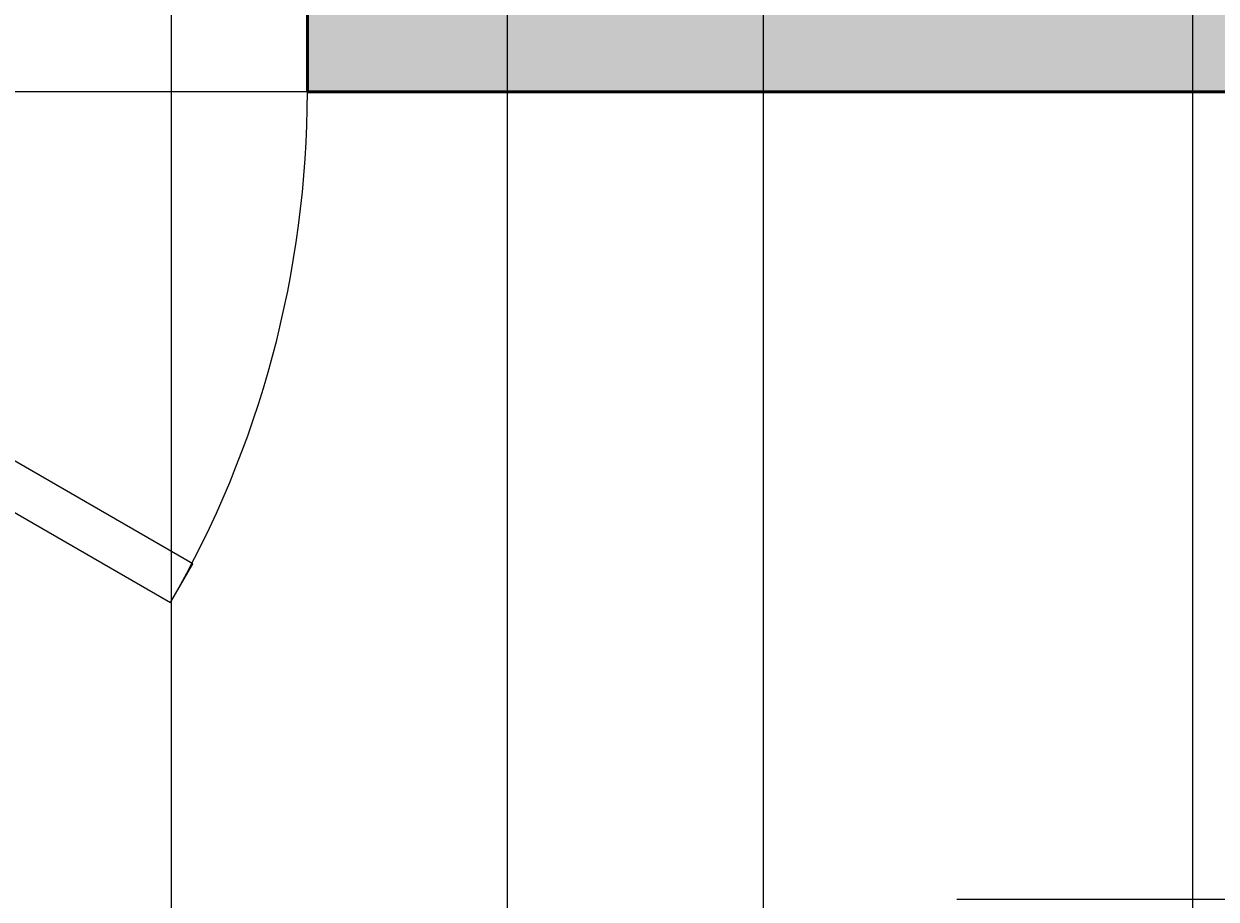
# Model space of a CAD drawing. Units: inches. Extents: x 2231 to 2461, y 2045 to 2455.
# Tile 27 of 95: x 2326 to 2361, y 2159 to 2185. Entities that reach past the tile are written whole.
import ezdxf

# ---------------------------------------------------------------- set-up
doc = ezdxf.new("R2010")
doc.units = ezdxf.units.IN
for name, color, linetype, lineweight in [('A-ANNO-DIMS', 2, 'Continuous', 18), ('A-DOOR', 3, 'Continuous', 25), ('A-WALL', 7, 'Continuous', 50)]:
    doc.layers.add(name, color=color, linetype=linetype, lineweight=lineweight)
doc.layers.add('A-WALL-PATT', color=18, linetype='Continuous', lineweight=13, true_color=0x000000)
doc.styles.get("Standard").update_dxf_attribs({"font": 'arial.ttf'})
doc.dimstyles.get("Standard").update_dxf_attribs({"dimtxt": 0.18, "dimasz": 0.18, "dimexe": 0.18, "dimexo": 0.0625, "dimgap": 0.09, "dimtad": 0, "dimtih": 1, "dimtoh": 1, "dimdec": 4, "dimzin": 0, "dimdsep": 46, "dimtxsty": 'Standard', "dimcen": 0.09, "dimadec": 0, "dimazin": 0, "dimtfac": 1, "dimtdec": 4, "dimtofl": 0, "dimtmove": 0, "dimatfit": 3, "dimfxl": 1, "dimtolj": 1, "dimtzin": 0, "dimarcsym": 0})

# ---------------------------------------------------------------- blocks, each defined once
blk = doc.blocks.new('*U4')
for p, q in [((0, 0), (0, 6)), ((40, 0), (40, 6))]:
    blk.add_line(p, q)
blk.add_lwpolyline([(0, 0), (34.641, -20), (35.516, -18.484), (0.875, 1.516)], close=True)
blk.add_arc((0, 0), 40, 330, 0)
blk = doc.blocks.new('*D50')
at = {"layer": 'A-ANNO-DIMS', "color": 0, "lineweight": -2, "transparency": 16777216}
for p, q in [((2304.794, 2182.895), (2304.794, 2454.645)), ((2334.794, 2182.895), (2334.794, 2454.645)), ((2304.974, 2454.465), (2319.575, 2454.465)), ((2334.614, 2454.465), (2320.012, 2454.465))]:
    blk.add_line(p, q, dxfattribs=at)
at = {"layer": 'A-ANNO-DIMS', "color": 0, "transparency": 16777216}
for points in [[(2304.974, 2454.495), (2304.974, 2454.435), (2304.794, 2454.465)], [(2334.614, 2454.495), (2334.614, 2454.435), (2334.794, 2454.465)]]:
    blk.add_solid(points, dxfattribs=at)
at = {"layer": 'Defpoints', "color": 0, "transparency": 16777216}
for p in [(2334.794, 2454.465), (2304.794, 2182.833), (2334.794, 2182.833)]:
    blk.add_point(p, dxfattribs=at)
at = {"layer": 'A-ANNO-DIMS', "color": 0, "transparency": 16777216, "insert": (2319.794, 2454.465), "char_height": 0.18, "attachment_point": 5}
blk.add_mtext('\\A1;30', dxfattribs=at)
blk = doc.blocks.new('*D51')
at = {"layer": 'A-ANNO-DIMS', "color": 0, "lineweight": -2, "transparency": 16777216}
for p, q in [((2258.794, 2306.77), (2258.794, 2044.803)), ((2330.794, 2306.77), (2330.794, 2044.803)), ((2258.974, 2044.983), (2294.576, 2044.983)), ((2330.614, 2044.983), (2295.011, 2044.983))]:
    blk.add_line(p, q, dxfattribs=at)
at = {"layer": 'A-ANNO-DIMS', "color": 0, "transparency": 16777216}
for points in [[(2258.974, 2045.013), (2258.974, 2044.953), (2258.794, 2044.983)], [(2330.614, 2045.013), (2330.614, 2044.953), (2330.794, 2044.983)]]:
    blk.add_solid(points, dxfattribs=at)
at = {"layer": 'Defpoints', "color": 0, "transparency": 16777216}
for p in [(2258.794, 2306.833), (2330.794, 2306.833), (2330.794, 2044.983)]:
    blk.add_point(p, dxfattribs=at)
at = {"layer": 'A-ANNO-DIMS', "color": 0, "transparency": 16777216, "insert": (2294.794, 2044.983), "char_height": 0.18, "attachment_point": 5}
blk.add_mtext('\\A1;72', dxfattribs=at)
blk = doc.blocks.new('*D52')
at = {"layer": 'A-ANNO-DIMS', "color": 0, "lineweight": -2, "transparency": 16777216}
for p, q in [((2330.794, 2306.77), (2330.794, 2044.803)), ((2360.794, 2306.77), (2360.794, 2044.803)), ((2330.974, 2044.983), (2345.575, 2044.983)), ((2360.614, 2044.983), (2346.012, 2044.983))]:
    blk.add_line(p, q, dxfattribs=at)
at = {"layer": 'A-ANNO-DIMS', "color": 0, "transparency": 16777216}
for points in [[(2330.974, 2045.013), (2330.974, 2044.953), (2330.794, 2044.983)], [(2360.614, 2045.013), (2360.614, 2044.953), (2360.794, 2044.983)]]:
    blk.add_solid(points, dxfattribs=at)
at = {"layer": 'Defpoints', "color": 0, "transparency": 16777216}
for p in [(2330.794, 2306.833), (2360.794, 2306.833), (2360.794, 2044.983)]:
    blk.add_point(p, dxfattribs=at)
at = {"layer": 'A-ANNO-DIMS', "color": 0, "transparency": 16777216, "insert": (2345.794, 2044.983), "char_height": 0.18, "attachment_point": 5}
blk.add_mtext('\\A1;30', dxfattribs=at)
blk = doc.blocks.new('*D60')
at = {"layer": 'A-ANNO-DIMS', "color": 0, "lineweight": -2, "transparency": 16777216}
for p, q in [((2432.731, 2182.833), (2230.981, 2182.833)), ((2231.161, 2182.653), (2231.161, 2166.906)), ((2231.161, 2150.795), (2231.161, 2166.542)), ((2432.731, 2150.615), (2230.981, 2150.615))]:
    blk.add_line(p, q, dxfattribs=at)
at = {"layer": 'A-ANNO-DIMS', "color": 0, "transparency": 16777216}
for points in [[(2231.131, 2182.653), (2231.191, 2182.653), (2231.161, 2182.833)], [(2231.131, 2150.795), (2231.191, 2150.795), (2231.161, 2150.615)]]:
    blk.add_solid(points, dxfattribs=at)
at = {"layer": 'Defpoints', "color": 0, "transparency": 16777216}
for p in [(2231.161, 2182.833), (2432.794, 2182.833), (2432.794, 2150.615)]:
    blk.add_point(p, dxfattribs=at)
at = {"layer": 'A-ANNO-DIMS', "color": 0, "transparency": 16777216, "insert": (2231.161, 2166.724), "char_height": 0.18, "attachment_point": 5}
blk.add_mtext('\\A1;32.22', dxfattribs=at)
blk = doc.blocks.new('*D65')
at = {"layer": 'A-ANNO-DIMS', "color": 0, "lineweight": -2, "transparency": 16777216}
for p, q in [((2285.635, 2189.285), (2285.635, 2044.803)), ((2340.667, 2189.285), (2340.667, 2044.803)), ((2285.815, 2044.983), (2312.758, 2044.983)), ((2340.487, 2044.983), (2313.545, 2044.983))]:
    blk.add_line(p, q, dxfattribs=at)
at = {"layer": 'A-ANNO-DIMS', "color": 0, "transparency": 16777216}
for points in [[(2285.815, 2045.013), (2285.815, 2044.953), (2285.635, 2044.983)], [(2340.487, 2045.013), (2340.487, 2044.953), (2340.667, 2044.983)]]:
    blk.add_solid(points, dxfattribs=at)
at = {"layer": 'Defpoints', "color": 0, "transparency": 16777216}
for p in [(2285.635, 2189.348), (2340.667, 2189.348), (2340.667, 2044.983)]:
    blk.add_point(p, dxfattribs=at)
at = {"layer": 'A-ANNO-DIMS', "color": 0, "transparency": 16777216, "insert": (2313.151, 2044.983), "char_height": 0.18, "attachment_point": 5}
blk.add_mtext('\\A1;55.03', dxfattribs=at)
blk = doc.blocks.new('*D66')
at = {"layer": 'A-ANNO-DIMS', "color": 0, "lineweight": -2, "transparency": 16777216}
for p, q in [((2348.189, 2096.895), (2348.189, 2454.645)), ((2408.794, 2096.895), (2408.794, 2454.645)), ((2348.369, 2454.465), (2378.167, 2454.465)), ((2408.614, 2454.465), (2378.815, 2454.465))]:
    blk.add_line(p, q, dxfattribs=at)
at = {"layer": 'A-ANNO-DIMS', "color": 0, "transparency": 16777216}
for points in [[(2348.369, 2454.495), (2348.369, 2454.435), (2348.189, 2454.465)], [(2408.614, 2454.495), (2408.614, 2454.435), (2408.794, 2454.465)]]:
    blk.add_solid(points, dxfattribs=at)
at = {"layer": 'Defpoints', "color": 0, "transparency": 16777216}
for p in [(2408.794, 2454.465), (2348.189, 2096.833), (2408.794, 2096.833)]:
    blk.add_point(p, dxfattribs=at)
at = {"layer": 'A-ANNO-DIMS', "color": 0, "transparency": 16777216, "insert": (2378.491, 2454.465), "char_height": 0.18, "attachment_point": 5}
blk.add_mtext('\\A1;60.6', dxfattribs=at)
blk = doc.blocks.new('*D69')
at = {"layer": 'A-ANNO-DIMS', "color": 0, "lineweight": -2, "transparency": 16777216}
for p, q in [((2340.667, 2189.285), (2340.667, 2044.803)), ((2394.794, 2186.77), (2394.794, 2044.803)), ((2340.847, 2044.983), (2367.337, 2044.983)), ((2394.614, 2044.983), (2368.124, 2044.983))]:
    blk.add_line(p, q, dxfattribs=at)
at = {"layer": 'A-ANNO-DIMS', "color": 0, "transparency": 16777216}
for points in [[(2340.847, 2045.013), (2340.847, 2044.953), (2340.667, 2044.983)], [(2394.614, 2045.013), (2394.614, 2044.953), (2394.794, 2044.983)]]:
    blk.add_solid(points, dxfattribs=at)
at = {"layer": 'Defpoints', "color": 0, "transparency": 16777216}
for p in [(2340.667, 2189.348), (2394.794, 2186.833), (2394.794, 2044.983)]:
    blk.add_point(p, dxfattribs=at)
at = {"layer": 'A-ANNO-DIMS', "color": 0, "transparency": 16777216, "insert": (2367.73, 2044.983), "char_height": 0.18, "attachment_point": 5}
blk.add_mtext('\\A1;54.13', dxfattribs=at)
blk = doc.blocks.new('*D73')
at = {"layer": 'A-ANNO-DIMS', "color": 0, "lineweight": -2, "transparency": 16777216}
for p, q in [((2334.856, 2182.833), (2460.606, 2182.833)), ((2460.426, 2182.653), (2460.426, 2171.156)), ((2460.426, 2159.295), (2460.426, 2170.792)), ((2353.872, 2159.115), (2460.606, 2159.115))]:
    blk.add_line(p, q, dxfattribs=at)
at = {"layer": 'A-ANNO-DIMS', "color": 0, "transparency": 16777216}
for points in [[(2460.396, 2182.653), (2460.456, 2182.653), (2460.426, 2182.833)], [(2460.396, 2159.295), (2460.456, 2159.295), (2460.426, 2159.115)]]:
    blk.add_solid(points, dxfattribs=at)
at = {"layer": 'Defpoints', "color": 0, "transparency": 16777216}
for p in [(2334.794, 2182.833), (2460.426, 2182.833), (2353.809, 2159.115)]:
    blk.add_point(p, dxfattribs=at)
at = {"layer": 'A-ANNO-DIMS', "color": 0, "transparency": 16777216, "insert": (2460.426, 2170.974), "char_height": 0.18, "attachment_point": 5}
blk.add_mtext('\\A1;23.717', dxfattribs=at)

msp = doc.modelspace()

# ---------------------------------------------------------------- hatches: boundary and pattern name
at = {"layer": 'A-WALL-PATT'}
h = msp.add_hatch(color=256, dxfattribs=at)
h.dxf.hatch_style = 1
h.paths.add_polyline_path([(2441.7935, 2269.1535), (2432.7935, 2269.1535), (2432.7935, 2186.8328), (2396.7935, 2186.8328), (2396.7935, 2286.8328), (2394.7935, 2286.8328), (2394.7935, 2186.8328), (2334.7935, 2186.8328), (2334.7935, 2182.8328), (2432.7935, 2182.8328), (2432.7935, 2072.8328), (2416.6639, 2072.8328), (2416.6639, 2063.8328), (2441.7935, 2063.8328)])
h.paths.add_polyline_path([(2368.6639, 2072.8328), (2367.04, 2072.8328), (2330.7942, 2072.8328), (2330.7397, 2063.8328), (2368.6639, 2063.8328)])
h.paths.add_polyline_path([(2300.7392, 2068.3328), (2300.7392, 2072.8328), (2298.7935, 2072.8328), (2294.7935, 2072.8328), (2258.7935, 2072.8328), (2258.7935, 2120.8328), (2294.7935, 2120.8328), (2298.7935, 2120.8328), (2298.7935, 2128.8328), (2294.7935, 2128.8328), (2294.7935, 2124.8328), (2258.7935, 2124.8328), (2258.7935, 2182.8328), (2294.7935, 2182.8328), (2294.7935, 2174.8328), (2298.7935, 2174.8328), (2298.7935, 2182.8328), (2304.7935, 2182.8328), (2304.7935, 2186.8328), (2258.7935, 2186.8328), (2258.7935, 2221.999), (2249.7935, 2221.999), (2249.7935, 2063.8328), (2300.7392, 2063.8328)])
h.paths.add_polyline_path([(2391.9338, 2435.8328), (2333.82, 2435.8328), (2333.82, 2426.8328), (2368.7935, 2426.8328), (2368.7935, 2374.9508), (2368.7935, 2370.8328), (2372.3935, 2370.8328), (2372.7935, 2370.8328), (2372.7935, 2426.8328), (2391.9338, 2426.8328)])
h.paths.add_polyline_path([(2441.7935, 2435.8328), (2415.9338, 2435.8328), (2415.9338, 2426.8328), (2432.7935, 2426.8328), (2432.7935, 2334.8328), (2372.7935, 2334.8328), (2372.7935, 2346.8328), (2368.7935, 2346.8328), (2368.7935, 2306.8328), (2360.7935, 2306.8328), (2360.7935, 2302.8328), (2368.7935, 2302.8328), (2372.7935, 2302.8328), (2372.7935, 2330.8328), (2432.7935, 2330.8328), (2432.7935, 2317.1535), (2441.7935, 2317.1535)])
h.paths.add_polyline_path([(2285.82, 2435.8328), (2249.7935, 2435.8328), (2249.7935, 2269.999), (2258.7935, 2269.999), (2258.7935, 2302.8328), (2318.8168, 2302.8328), (2330.7935, 2302.8328), (2330.7935, 2306.8328), (2258.7935, 2306.8328), (2258.7935, 2426.8328), (2285.82, 2426.8328)])

# ---------------------------------------------------------------- linework, layer by layer
at = {"layer": 'A-WALL'}
for q in [(2334.7935, 2186.8328), (2432.7935, 2182.8328)]:
    msp.add_line((2334.7935, 2182.8328), q, dxfattribs=at)

# ---------------------------------------------------------------- block references
at = {"layer": 'A-DOOR', "xscale": 0.75, "yscale": 0.75, "zscale": 0.75}
msp.add_blockref('*U4', (2304.7935, 2182.8328), dxfattribs=at)

# ---------------------------------------------------------------- dimensions: what is measured, and where the dimension line sits
at = {"layer": 'A-ANNO-DIMS'}
for base, p1, p2, override, picture, middle in [((2334.7935, 2454.4653), (2304.7935, 2182.8328), (2334.7935, 2182.8328), {"dimdec": 0, "dimlfac": 1, "dimrnd": 0, "dimzin": 0, "dimdsep": 46, "dimlunit": 2}, '*D50', (2319.7935, 2454.4653)), ((2408.7935, 2454.4653), (2348.1888, 2096.8328), (2408.7935, 2096.8328), {"dimdec": 1, "dimlfac": 1, "dimrnd": 0, "dimzin": 0, "dimdsep": 46, "dimlunit": 2}, '*D66', (2378.4912, 2454.4653)), ((2330.7935, 2044.9825), (2258.7935, 2306.8328), (2330.7935, 2306.8328), {"dimdec": 0, "dimlfac": 1, "dimrnd": 0, "dimzin": 0, "dimdsep": 46, "dimlunit": 2}, '*D51', (2294.7935, 2044.9825)), ((2360.7935, 2044.9825), (2330.7935, 2306.8328), (2360.7935, 2306.8328), {"dimdec": 0, "dimlfac": 1, "dimrnd": 0, "dimzin": 0, "dimdsep": 46, "dimlunit": 2}, '*D52', (2345.7935, 2044.9825)), ((2340.6673, 2044.9825), (2285.6353, 2189.3477), (2340.6673, 2189.3477), {"dimdec": 2, "dimlfac": 1, "dimrnd": 0, "dimzin": 0, "dimdsep": 46, "dimlunit": 2}, '*D65', (2313.1513, 2044.9825)), ((2394.7935, 2044.9825), (2340.6673, 2189.3477), (2394.7935, 2186.8328), {"dimdec": 2, "dimlfac": 1, "dimrnd": 0, "dimzin": 0, "dimdsep": 46, "dimlunit": 2}, '*D69', (2367.7304, 2044.9825))]:
    dim = msp.add_linear_dim(base=base, p1=p1, p2=p2, dimstyle='Standard', override=override, dxfattribs=at)
    dim.commit()
    dim.dimension.update_dxf_attribs({"geometry": picture, "text_midpoint": middle})
for base, p1, p2, override, picture, middle in [((2231.161, 2182.8328), (2432.7935, 2150.6145), (2432.7935, 2182.8328), {"dimdec": 2, "dimlfac": 1, "dimrnd": 0, "dimzin": 0, "dimdsep": 46, "dimlunit": 2}, '*D60', (2231.161, 2166.7237)), ((2460.426, 2182.8328), (2353.8091, 2159.1154), (2334.7935, 2182.8328), {"dimdec": 3, "dimlfac": 1, "dimrnd": 0, "dimzin": 0, "dimdsep": 46, "dimlunit": 2}, '*D73', (2460.426, 2170.9741))]:
    dim = msp.add_linear_dim(base=base, p1=p1, p2=p2, angle=90, dimstyle='Standard', override=override, dxfattribs=at)
    dim.commit()
    dim.dimension.update_dxf_attribs({"geometry": picture, "text_midpoint": middle})

doc.saveas('drawing.dxf')
